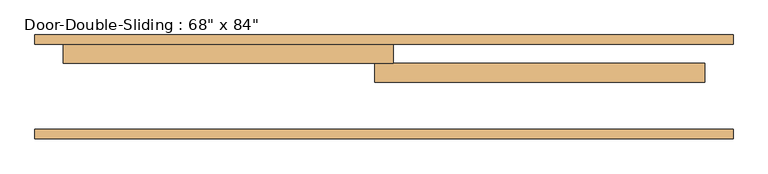
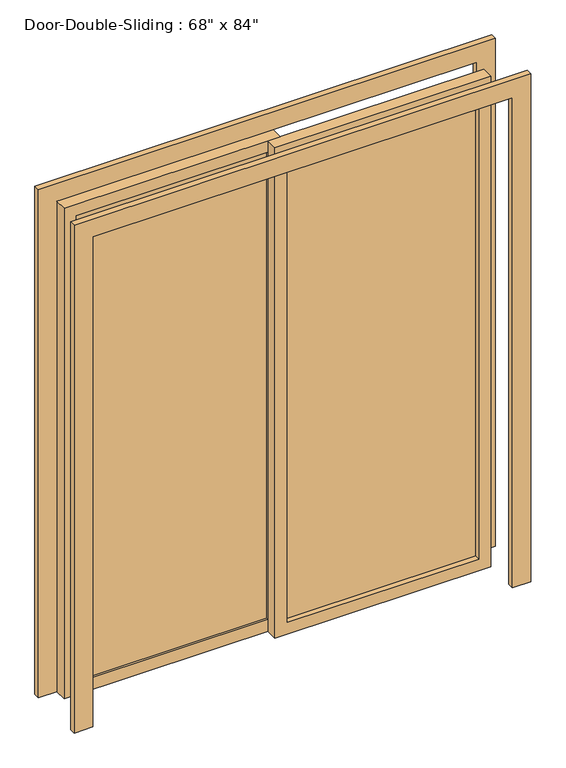
"""IFC4 building model written with IfcOpenShell, lengths in millimetres: door geometry."""

from ifc_helpers import new_model, si_unit, frame, origin, place, context, project, spatial, polyline, outline, extrude, source, transform, mapped, element, save


def door_45189e27(model_context):
    return source(origin(), model_context, "Body", "SweptSolid", [
        extrude(outline(polyline([(0.0, 939.8), (2209.8, 939.8), (2209.8, -939.8), (0.0, -939.8), (0.0, -863.6), (2133.6, -863.6), (2133.6, 863.6), (0.0, 863.6), (0.0, 939.8)])), frame((0.0, 241.3, 0.0), z_axis=(0.0, 1.0, 0.0), x_axis=(0.0, 0.0, 1.0)), (0.0, 0.0, 1.0), 25.4),
        extrude(outline(polyline([(0.0, -939.8), (0.0, -863.6), (2133.6, -863.6), (2133.6, 863.6), (0.0, 863.6), (0.0, 939.8), (2209.8, 939.8), (2209.8, -939.8), (0.0, -939.8)])), frame((0.0, -12.7, 0.0), z_axis=(0.0, 1.0, 0.0), x_axis=(0.0, 0.0, 1.0)), (0.0, 0.0, 1.0), 25.4),
        extrude(outline(polyline([(2133.6, 25.4), (2133.6, -863.6), (0.0, -863.6), (0.0, 25.4), (2133.6, 25.4)]), holes=[polyline([(2082.8, -25.4), (50.8, -25.4), (50.8, -812.8), (2082.8, -812.8), (2082.8, -25.4)])]), frame((0.0, 190.5, 0.0), z_axis=(0.0, 1.0, 0.0), x_axis=(0.0, 0.0, 1.0)), (0.0, 0.0, 1.0), 50.8),
        extrude(outline(polyline([(2133.6, -25.4), (0.0, -25.4), (0.0, 863.6), (2133.6, 863.6), (2133.6, -25.4)]), holes=[polyline([(2082.8, 25.4), (2082.8, 812.8), (50.8, 812.8), (50.8, 25.4), (2082.8, 25.4)])]), frame((0.0, 139.7, 0.0), z_axis=(0.0, 1.0, 0.0), x_axis=(0.0, 0.0, 1.0)), (0.0, 0.0, 1.0), 50.8),
        extrude(outline(polyline([(-25.4, 200.025), (-812.8, 200.025), (-812.8, 206.375), (-25.4, 206.375), (-25.4, 200.025)])), frame((0.0, 0.0, 50.8), z_axis=(0.0, 0.0, 1.0), x_axis=(1.0, 0.0, 0.0)), (0.0, 0.0, 1.0), 2032.0),
        extrude(outline(polyline([(25.4, 168.275), (812.8, 168.275), (812.8, 161.925), (25.4, 161.925), (25.4, 168.275)])), frame((0.0, 0.0, 50.8), z_axis=(0.0, 0.0, 1.0), x_axis=(1.0, 0.0, 0.0)), (0.0, 0.0, 1.0), 2032.0),
    ])


if __name__ == "__main__":
    model = new_model("IFC4")
    model_context = context("Model", 3, world=origin())
    ifc_project = project(units=[si_unit("LENGTHUNIT", "METRE", prefix="MILLI")], contexts=[model_context])
    site = spatial("IfcSite", under=ifc_project)
    building = spatial("IfcBuilding", under=site)
    placement = place(None, origin())
    door_shape = door_45189e27(model_context)
    element("IfcDoor", 1, ObjectType="Door-Double-Sliding : 68\" x 84\"", at=placement, inside=building, context=model_context, shape_type="MappedRepresentation", body=[
        mapped(door_shape, transform((0.0, 0.0, 0.0), x_axis=(1.0, 0.0, 0.0), y_axis=(0.0, 1.0, 0.0), z_axis=(0.0, 0.0, 1.0))),
    ])
    save(model, "model.ifc")

# Revit data of these elements
# Type "Door-Double-Sliding : 68\" x 84\""
#   Type Mark = "9"
#   Construction Type Id = "opn-d45"
#   Assembly Code = "C1020"
#   Analytic Construction = "Wood frame, double glass door "
#   Thickness = 0' - 2"
#   Thermal Resistance (R) = 1.8150 (h·ft²·°F)/BTU
#   Heat Transfer Coefficient (U) = 0.5510 BTU/(h·ft²·°F)
#   Height = 7' - 0"
#   Rail Width = 0' - 2"
#   Stiles = 0' - 2"
#   Trim Projection Ext = 0' - 1"
#   Trim Projection Int = 0' - 1"
#   Trim Width = 0' - 3"
#   Width = 5' - 8"
#   Define Thermal Properties by = 1
#   Glazing = Glass
#   Panel Material = Wood - Birch - Solid Stained Light Low Gloss
#   Trim Material = Paint - Sienna
#   Visual Light Transmittance = 0
#   Solar Heat Gain Coefficient = 0
#   Function = (empty or 0)
#   Wall Closure = (empty or 0)
# Element 1 (IfcDoor, "Door-Double-Sliding : 68\" x 84\"")
#   Materials on its faces: "Paint - Sienna", "Wood - Birch - Solid Stained Light Low Gloss", "Glass"
# Materials
#   "Glass": class "Glass", colour RGB 0 128 192, transparency 0.75, Description = "Soda Lime Glass", Cost = 0
#   "Wood - Birch - Solid Stained Light Low Gloss": class "Wood", colour RGB 210 159 95, transparency 0, Cost = 0
#   "Paint - Sienna": colour RGB 118 70 51, transparency 0, Cost = 0
